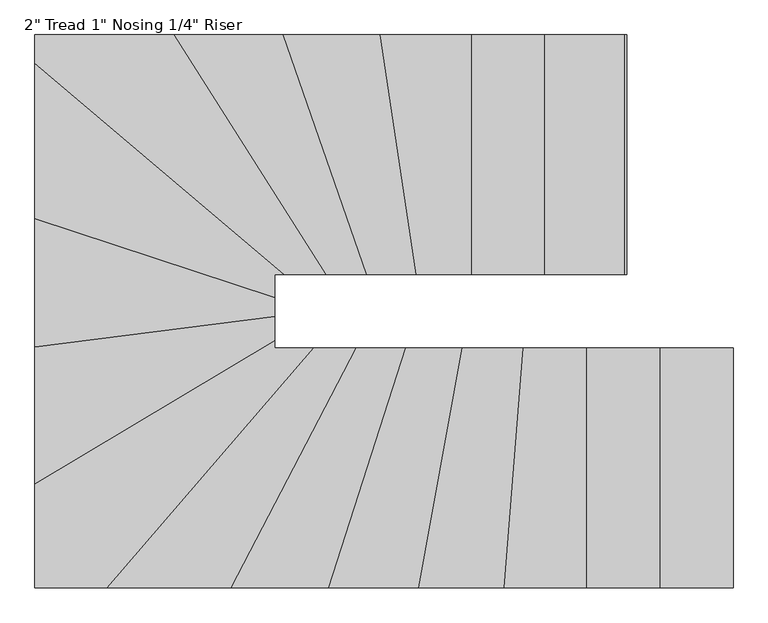
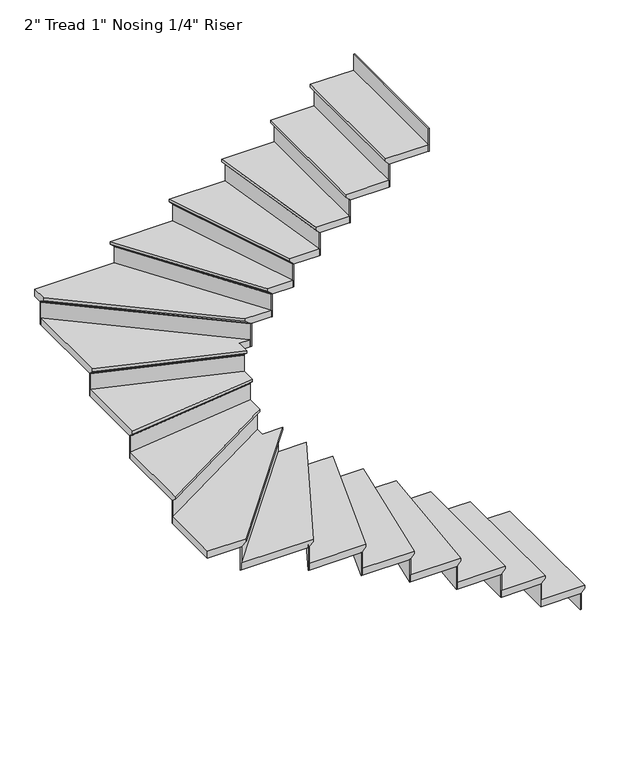
"""IFC4 building model written with IfcOpenShell, lengths in millimetres: stair flight geometry."""

from ifc_helpers import new_model, si_unit, origin, place, context, project, spatial, faceted_brep, source, transform, mapped, element, save


def stair_flight_79a896a8(model_context):
    return source(origin(), model_context, "Body", "Brep", [
        faceted_brep([(-8086.227471, 3122.5174997, 150.2833333), (-8086.227471, 3122.5174997, 169.3333333), (-8086.227471, 2208.1174997, 169.3333333), (-8086.227471, 2208.1174997, 150.2833333), (-8111.627471, 3122.5174997, 124.8833333), (-8111.627471, 2208.1174997, 124.8833333), (-8391.027471, 3122.5174997, 169.3333333), (-8391.027471, 2208.1174997, 169.3333333), (-8111.627471, 2208.1174997, 118.5333333), (-8391.027471, 2208.1174997, 118.5333333), (-8391.027471, 3122.5174997, 118.5333333), (-8111.627471, 3122.5174997, 118.5333333)], [[[0, 1, 2, 3]], [[4, 0, 3, 5]], [[2, 1, 6, 7]], [[8, 9, 10, 11]], [[2, 7, 9, 8, 5, 3]], [[8, 11, 4, 5]], [[6, 1, 0, 4, 11, 10]], [[7, 6, 10, 9]]]),
        faceted_brep([(-8111.627471, 3122.5174997, 118.5333333), (-8111.627471, 3122.5174997, 0.0), (-8117.977471, 3122.5174997, 0.0), (-8117.977471, 3122.5174997, 118.5333333), (-8111.627471, 2208.1174997, 118.5333333), (-8117.977471, 2208.1174997, 118.5333333), (-8117.977471, 2208.1174997, 0.0), (-8111.627471, 2208.1174997, 0.0)], [[[0, 1, 2, 3]], [[4, 5, 6, 7]], [[1, 0, 4, 7]], [[2, 1, 7, 6]], [[3, 2, 6, 5]], [[0, 3, 5, 4]]]),
        faceted_brep([(-8391.027471, 3122.5174997, 287.8666667), (-8391.027471, 3122.5174997, 118.5333333), (-8397.377471, 3122.5174997, 118.5333333), (-8397.377471, 3122.5174997, 287.8666667), (-8391.027471, 2208.1174997, 287.8666667), (-8397.377471, 2208.1174997, 287.8666667), (-8397.377471, 2208.1174997, 118.5333333), (-8391.027471, 2208.1174997, 118.5333333)], [[[0, 1, 2, 3]], [[4, 5, 6, 7]], [[1, 0, 4, 7]], [[2, 1, 7, 6]], [[3, 2, 6, 5]], [[0, 3, 5, 4]]]),
        faceted_brep([(-8365.627471, 2208.1174997, 338.6666667), (-8365.627471, 3122.5174997, 338.6666667), (-8670.427471, 3122.5174997, 338.6666667), (-8670.427471, 2208.1174997, 338.6666667), (-8391.027471, 2208.1174997, 287.8666667), (-8670.427471, 2208.1174997, 287.8666667), (-8670.427471, 3122.5174997, 287.8666667), (-8391.027471, 3122.5174997, 287.8666667), (-8391.027471, 2208.1174997, 294.2166667), (-8365.627471, 2208.1174997, 319.6166667), (-8391.027471, 3122.5174997, 294.2166667), (-8365.627471, 3122.5174997, 319.6166667)], [[[0, 1, 2, 3]], [[4, 5, 6, 7]], [[0, 3, 5, 4, 8, 9]], [[4, 7, 10, 8]], [[2, 1, 11, 10, 7, 6]], [[3, 2, 6, 5]], [[11, 1, 0, 9]], [[10, 11, 9, 8]]]),
        faceted_brep([(-8670.427471, 3122.5174997, 457.2), (-8670.427471, 3122.5174997, 287.8666667), (-8676.777471, 3122.5174997, 287.8666667), (-8676.777471, 3122.5174997, 457.2), (-8670.427471, 2208.1174997, 457.2), (-8676.777471, 2208.1174997, 457.2), (-8676.777471, 2208.1174997, 287.8666667), (-8670.427471, 2208.1174997, 287.8666667)], [[[0, 1, 2, 3]], [[4, 5, 6, 7]], [[1, 0, 4, 7]], [[2, 1, 7, 6]], [[3, 2, 6, 5]], [[0, 3, 5, 4]]]),
        faceted_brep([(-8645.027471, 2208.1174997, 508.0), (-8645.027471, 3122.5174997, 508.0), (-8913.9170004, 3122.5174997, 508.0), (-8985.895083, 2208.1174997, 508.0), (-8670.427471, 2208.1174997, 457.2), (-8985.895083, 2208.1174997, 457.2), (-8913.9170004, 3122.5174997, 457.2), (-8670.427471, 3122.5174997, 457.2), (-8670.427471, 2208.1174997, 463.55), (-8645.027471, 2208.1174997, 488.95), (-8670.427471, 3122.5174997, 463.55), (-8645.027471, 3122.5174997, 488.95)], [[[0, 1, 2, 3]], [[4, 5, 6, 7]], [[0, 3, 5, 4, 8, 9]], [[4, 7, 10, 8]], [[2, 1, 11, 10, 7, 6]], [[3, 2, 6, 5]], [[11, 1, 0, 9]], [[10, 11, 9, 8]]]),
        faceted_brep([(-8913.9170004, 3122.5174997, 626.5333333), (-8913.9170004, 3122.5174997, 457.2), (-8920.2866431, 3122.5174997, 457.2), (-8920.2866431, 3122.5174997, 626.5333333), (-8985.895083, 2208.1174997, 626.5333333), (-8992.2647257, 2208.1174997, 626.5333333), (-8992.2647257, 2208.1174997, 457.2), (-8985.895083, 2208.1174997, 457.2)], [[[0, 1, 2, 3]], [[4, 5, 6, 7]], [[1, 0, 4, 7]], [[2, 1, 7, 6]], [[3, 2, 6, 5]], [[0, 3, 5, 4]]]),
        faceted_brep([(-8960.4165123, 2208.1174997, 677.3333333), (-8888.4384297, 3122.5174997, 677.3333333), (-9146.6716343, 3122.5174997, 677.3333333), (-9312.6130409, 2208.1174997, 677.3333333), (-8985.895083, 2208.1174997, 626.5333333), (-9312.6130409, 2208.1174997, 626.5333333), (-9146.6716343, 3122.5174997, 626.5333333), (-8913.9170004, 3122.5174997, 626.5333333), (-8985.895083, 2208.1174997, 632.8833333), (-8960.4165123, 2208.1174997, 658.2833333), (-8913.9170004, 3122.5174997, 632.8833333), (-8888.4384297, 3122.5174997, 658.2833333)], [[[0, 1, 2, 3]], [[4, 5, 6, 7]], [[0, 3, 5, 4, 8, 9]], [[4, 7, 10, 8]], [[2, 1, 11, 10, 7, 6]], [[3, 2, 6, 5]], [[11, 1, 0, 9]], [[10, 11, 9, 8]]]),
        faceted_brep([(-9146.6716343, 3122.5174997, 795.8666667), (-9146.6716343, 3122.5174997, 626.5333333), (-9153.125351, 3122.5174997, 626.5333333), (-9153.125351, 3122.5174997, 795.8666667), (-9312.6130409, 2208.1174997, 795.8666667), (-9319.0667575, 2208.1174997, 795.8666667), (-9319.0667575, 2208.1174997, 626.5333333), (-9312.6130409, 2208.1174997, 626.5333333)], [[[0, 1, 2, 3]], [[4, 5, 6, 7]], [[1, 0, 4, 7]], [[2, 1, 7, 6]], [[3, 2, 6, 5]], [[0, 3, 5, 4]]]),
        faceted_brep([(-9286.7981743, 2208.1174997, 846.6666667), (-9120.8567677, 3122.5174997, 846.6666667), (-9363.0169479, 3122.5174997, 846.6666667), (-9656.7954295, 2208.1174997, 846.6666667), (-9312.6130409, 2208.1174997, 795.8666667), (-9656.7954295, 2208.1174997, 795.8666667), (-9363.0169479, 3122.5174997, 795.8666667), (-9146.6716343, 3122.5174997, 795.8666667), (-9312.6130409, 2208.1174997, 802.2166667), (-9286.7981743, 2208.1174997, 827.6166667), (-9146.6716343, 3122.5174997, 802.2166667), (-9120.8567677, 3122.5174997, 827.6166667)], [[[0, 1, 2, 3]], [[4, 5, 6, 7]], [[0, 3, 5, 4, 8, 9]], [[4, 7, 10, 8]], [[2, 1, 11, 10, 7, 6]], [[3, 2, 6, 5]], [[11, 1, 0, 9]], [[10, 11, 9, 8]]]),
        faceted_brep([(-9363.0169479, 3122.5174997, 965.2), (-9363.0169479, 3122.5174997, 795.8666667), (-9369.6866273, 3122.5174997, 795.8666667), (-9369.6866273, 3122.5174997, 965.2), (-9656.7954295, 2208.1174997, 965.2), (-9663.4651089, 2208.1174997, 965.2), (-9663.4651089, 2208.1174997, 795.8666667), (-9656.7954295, 2208.1174997, 795.8666667)], [[[0, 1, 2, 3]], [[4, 5, 6, 7]], [[1, 0, 4, 7]], [[2, 1, 7, 6]], [[3, 2, 6, 5]], [[0, 3, 5, 4]]]),
        faceted_brep([(-9630.1167118, 2208.1174997, 1016.0), (-9336.3382302, 3122.5174997, 1016.0), (-9552.3693579, 3122.5174997, 1016.0), (-10030.2035425, 2208.1174997, 1016.0), (-9656.7954295, 2208.1174997, 965.2), (-10030.2035425, 2208.1174997, 965.2), (-9552.3693579, 3122.5174997, 965.2), (-9363.0169479, 3122.5174997, 965.2), (-9656.7954295, 2208.1174997, 971.55), (-9630.1167118, 2208.1174997, 996.95), (-9363.0169479, 3122.5174997, 971.55), (-9336.3382302, 3122.5174997, 996.95)], [[[0, 1, 2, 3]], [[4, 5, 6, 7]], [[0, 3, 5, 4, 8, 9]], [[4, 7, 10, 8]], [[2, 1, 11, 10, 7, 6]], [[3, 2, 6, 5]], [[11, 1, 0, 9]], [[10, 11, 9, 8]]]),
        faceted_brep([(-9552.3693579, 3122.5174997, 1134.5333333), (-9552.3693579, 3122.5174997, 965.2), (-9559.5341027, 3122.5174997, 965.2), (-9559.5341027, 3122.5174997, 1134.5333333), (-10030.2035425, 2208.1174997, 1134.5333333), (-10037.3682873, 2208.1174997, 1134.5333333), (-10037.3682873, 2208.1174997, 965.2), (-10030.2035425, 2208.1174997, 965.2)], [[[0, 1, 2, 3]], [[4, 5, 6, 7]], [[1, 0, 4, 7]], [[2, 1, 7, 6]], [[3, 2, 6, 5]], [[0, 3, 5, 4]]]),
        faceted_brep([(-10001.5445633, 2208.1174997, 1185.3333333), (-9523.7103787, 3122.5174997, 1185.3333333), (-9719.9061771, 3122.5174997, 1185.3333333), (-10506.0897865, 2208.1174997, 1185.3333333), (-10030.2035425, 2208.1174997, 1134.5333333), (-10506.0897865, 2208.1174997, 1134.5333333), (-9719.9061771, 3122.5174997, 1134.5333333), (-9552.3693579, 3122.5174997, 1134.5333333), (-10030.2035425, 2208.1174997, 1140.8833333), (-10001.5445633, 2208.1174997, 1166.2833333), (-9552.3693579, 3122.5174997, 1140.8833333), (-9523.7103787, 3122.5174997, 1166.2833333)], [[[0, 1, 2, 3]], [[4, 5, 6, 7]], [[0, 3, 5, 4, 8, 9]], [[4, 7, 10, 8]], [[2, 1, 11, 10, 7, 6]], [[3, 2, 6, 5]], [[11, 1, 0, 9]], [[10, 11, 9, 8]]]),
        faceted_brep([(-9719.9061771, 3122.5174997, 1303.8666667), (-9719.9061771, 3122.5174997, 1134.5333333), (-9728.2805322, 3122.5174997, 1134.5333333), (-9728.2805322, 3122.5174997, 1303.8666667), (-10506.0897865, 2208.1174997, 1303.8666667), (-10514.4641416, 2208.1174997, 1303.8666667), (-10514.4641416, 2208.1174997, 1134.5333333), (-10506.0897865, 2208.1174997, 1134.5333333)], [[[0, 1, 2, 3]], [[4, 5, 6, 7]], [[1, 0, 4, 7]], [[2, 1, 7, 6]], [[3, 2, 6, 5]], [[0, 3, 5, 4]]]),
        faceted_brep([(-10747.2073372, 2633.5177157, 1354.6666667), (-10747.2073372, 2208.1174997, 1354.6666667), (-10472.5923659, 2208.1174997, 1354.6666667), (-9686.4087566, 3122.5174997, 1354.6666667), (-9832.8073372, 3122.5174997, 1354.6666667), (-9832.8073372, 3181.4002288, 1354.6666667), (-10747.2073372, 2208.1174997, 1303.8666667), (-10747.2073372, 2633.5177157, 1303.8666667), (-9832.8073372, 3181.4002288, 1303.8666667), (-9832.8073372, 3122.5174997, 1303.8666667), (-9719.9061771, 3122.5174997, 1303.8666667), (-10506.0897865, 2208.1174997, 1303.8666667), (-9719.9061771, 3122.5174997, 1310.2166667), (-10506.0897865, 2208.1174997, 1310.2166667), (-9686.4087566, 3122.5174997, 1335.6166667), (-10472.5923659, 2208.1174997, 1335.6166667)], [[[0, 1, 2, 3, 4, 5]], [[6, 7, 8, 9, 10, 11]], [[1, 0, 7, 6]], [[11, 10, 12, 13]], [[5, 4, 9, 8]], [[0, 5, 8, 7]], [[14, 3, 2, 15]], [[12, 14, 15, 13]], [[2, 1, 6, 11, 13, 15]], [[4, 3, 14, 12, 10, 9]]]),
        faceted_brep([(-9832.8073372, 3181.4002288, 1473.2), (-9832.8073372, 3181.4002288, 1303.8666667), (-9832.8073372, 3188.8028327, 1303.8666667), (-9832.8073372, 3188.8028327, 1473.2), (-10747.2073372, 2633.5177157, 1473.2), (-10747.2073372, 2640.9203196, 1473.2), (-10747.2073372, 2640.9203196, 1303.8666667), (-10747.2073372, 2633.5177157, 1303.8666667)], [[[0, 1, 2, 3]], [[4, 5, 6, 7]], [[1, 0, 4, 7]], [[2, 1, 7, 6]], [[3, 2, 6, 5]], [[0, 3, 5, 4]]]),
        faceted_brep([(-10747.2073372, 2603.9073003, 1524.0), (-9832.8073372, 3151.7898134, 1524.0), (-9832.8073372, 3267.6146892, 1524.0), (-10747.2073372, 3151.2124555, 1524.0), (-10747.2073372, 2633.5177157, 1473.2), (-10747.2073372, 3151.2124555, 1473.2), (-9832.8073372, 3267.6146892, 1473.2), (-9832.8073372, 3181.4002288, 1473.2), (-10747.2073372, 2633.5177157, 1479.55), (-10747.2073372, 2603.9073003, 1504.95), (-9832.8073372, 3181.4002288, 1479.55), (-9832.8073372, 3151.7898134, 1504.95)], [[[0, 1, 2, 3]], [[4, 5, 6, 7]], [[0, 3, 5, 4, 8, 9]], [[4, 7, 10, 8]], [[2, 1, 11, 10, 7, 6]], [[3, 2, 6, 5]], [[11, 1, 0, 9]], [[10, 11, 9, 8]]]),
        faceted_brep([(-9832.8073372, 3267.6146892, 1642.5333333), (-9832.8073372, 3267.6146892, 1473.2), (-9832.8073372, 3274.0159334, 1473.2), (-9832.8073372, 3274.0159334, 1642.5333333), (-10747.2073372, 3151.2124555, 1642.5333333), (-10747.2073372, 3157.6136998, 1642.5333333), (-10747.2073372, 3157.6136998, 1473.2), (-10747.2073372, 3151.2124555, 1473.2)], [[[0, 1, 2, 3]], [[4, 5, 6, 7]], [[1, 0, 4, 7]], [[2, 1, 7, 6]], [[3, 2, 6, 5]], [[0, 3, 5, 4]]]),
        faceted_brep([(-10747.2073372, 3125.6074786, 1693.3333333), (-9832.8073372, 3242.0097122, 1693.3333333), (-9832.8073372, 3340.7509196, 1693.3333333), (-10747.2073372, 3641.8025654, 1693.3333333), (-10747.2073372, 3151.2124555, 1642.5333333), (-10747.2073372, 3641.8025654, 1642.5333333), (-9832.8073372, 3340.7509196, 1642.5333333), (-9832.8073372, 3267.6146892, 1642.5333333), (-10747.2073372, 3151.2124555, 1648.8833333), (-10747.2073372, 3125.6074786, 1674.2833333), (-9832.8073372, 3267.6146892, 1648.8833333), (-9832.8073372, 3242.0097122, 1674.2833333)], [[[0, 1, 2, 3]], [[4, 5, 6, 7]], [[0, 3, 5, 4, 8, 9]], [[4, 7, 10, 8]], [[2, 1, 11, 10, 7, 6]], [[3, 2, 6, 5]], [[11, 1, 0, 9]], [[10, 11, 9, 8]]]),
        faceted_brep([(-9832.8073372, 3340.7509196, 1811.8666667), (-9832.8073372, 3340.7509196, 1642.5333333), (-9832.8073372, 3347.4362214, 1642.5333333), (-9832.8073372, 3347.4362214, 1811.8666667), (-10747.2073372, 3641.8025654, 1811.8666667), (-10747.2073372, 3648.4878672, 1811.8666667), (-10747.2073372, 3648.4878672, 1642.5333333), (-10747.2073372, 3641.8025654, 1642.5333333)], [[[0, 1, 2, 3]], [[4, 5, 6, 7]], [[1, 0, 4, 7]], [[2, 1, 7, 6]], [[3, 2, 6, 5]], [[0, 3, 5, 4]]]),
        faceted_brep([(-10747.2073372, 3615.061358, 1862.6666667), (-9832.8073372, 3314.0097122, 1862.6666667), (-9832.8073372, 3401.9174997, 1862.6666667), (-9756.9168091, 3401.9174997, 1862.6666667), (-10747.2073372, 4242.112231, 1862.6666667), (-10747.2073372, 3641.8025654, 1811.8666667), (-10747.2073372, 4242.112231, 1811.8666667), (-9756.9168091, 3401.9174997, 1811.8666667), (-9832.8073372, 3401.9174997, 1811.8666667), (-9832.8073372, 3340.7509196, 1811.8666667), (-10747.2073372, 3641.8025654, 1818.2166667), (-10747.2073372, 3615.061358, 1843.6166667), (-9832.8073372, 3340.7509196, 1818.2166667), (-9832.8073372, 3314.0097122, 1843.6166667)], [[[0, 1, 2, 3, 4]], [[5, 6, 7, 8, 9]], [[0, 4, 6, 5, 10, 11]], [[5, 9, 12, 10]], [[2, 1, 13, 12, 9, 8]], [[4, 3, 7, 6]], [[13, 1, 0, 11]], [[12, 13, 11, 10]], [[3, 2, 8, 7]]]),
        faceted_brep([(-9756.9168091, 3401.9174997, 1981.2), (-9756.9168091, 3401.9174997, 1811.8666667), (-9747.1015867, 3401.9174997, 1811.8666667), (-9747.1015867, 3401.9174997, 1981.2), (-10747.2073372, 4242.112231, 1981.2), (-10747.2073372, 4250.4397852, 1981.2), (-10747.2073372, 4250.4397852, 1811.8666667), (-10747.2073372, 4242.112231, 1811.8666667)], [[[0, 1, 2, 3]], [[4, 5, 6, 7]], [[1, 0, 4, 7]], [[2, 1, 7, 6]], [[3, 2, 6, 5]], [[0, 3, 5, 4]]]),
        faceted_brep([(-10185.8825098, 4316.3174997, 2032.0), (-10747.2073372, 4316.3174997, 2032.0), (-10747.2073372, 4208.8020138, 2032.0), (-9796.1776986, 3401.9174997, 2032.0), (-9607.0675829, 3401.9174997, 2032.0), (-10747.2073372, 4316.3174997, 1981.2), (-10185.8825098, 4316.3174997, 1981.2), (-9607.0675829, 3401.9174997, 1981.2), (-9756.9168091, 3401.9174997, 1981.2), (-10747.2073372, 4242.112231, 1981.2), (-9756.9168091, 3401.9174997, 1987.55), (-10747.2073372, 4242.112231, 1987.55), (-9796.1776986, 3401.9174997, 2012.95), (-10747.2073372, 4208.8020138, 2012.95)], [[[0, 1, 2, 3, 4]], [[5, 6, 7, 8, 9]], [[1, 0, 6, 5]], [[9, 8, 10, 11]], [[4, 3, 12, 10, 8, 7]], [[0, 4, 7, 6]], [[12, 3, 2, 13]], [[10, 12, 13, 11]], [[2, 1, 5, 9, 11, 13]]]),
        faceted_brep([(-9607.0675829, 3401.9174997, 2150.5333333), (-9607.0675829, 3401.9174997, 1981.2), (-9599.552314, 3401.9174997, 1981.2), (-9599.552314, 3401.9174997, 2150.5333333), (-10185.8825098, 4316.3174997, 2150.5333333), (-10178.3672409, 4316.3174997, 2150.5333333), (-10178.3672409, 4316.3174997, 1981.2), (-10185.8825098, 4316.3174997, 1981.2)], [[[0, 1, 2, 3]], [[4, 5, 6, 7]], [[1, 0, 4, 7]], [[2, 1, 7, 6]], [[3, 2, 6, 5]], [[0, 3, 5, 4]]]),
        faceted_brep([(-10215.9435855, 4316.3174997, 2201.3333333), (-9637.1286586, 3401.9174997, 2201.3333333), (-9455.5314169, 3401.9174997, 2201.3333333), (-9774.3141998, 4316.3174997, 2201.3333333), (-10185.8825098, 4316.3174997, 2150.5333333), (-9774.3141998, 4316.3174997, 2150.5333333), (-9455.5314169, 3401.9174997, 2150.5333333), (-9607.0675829, 3401.9174997, 2150.5333333), (-10185.8825098, 4316.3174997, 2156.8833333), (-10215.9435855, 4316.3174997, 2182.2833333), (-9607.0675829, 3401.9174997, 2156.8833333), (-9637.1286586, 3401.9174997, 2182.2833333)], [[[0, 1, 2, 3]], [[4, 5, 6, 7]], [[0, 3, 5, 4, 8, 9]], [[4, 7, 10, 8]], [[2, 1, 11, 10, 7, 6]], [[3, 2, 6, 5]], [[11, 1, 0, 9]], [[10, 11, 9, 8]]]),
        faceted_brep([(-9455.5314169, 3401.9174997, 2319.8666667), (-9455.5314169, 3401.9174997, 2150.5333333), (-9448.8065916, 3401.9174997, 2150.5333333), (-9448.8065916, 3401.9174997, 2319.8666667), (-9774.3141998, 4316.3174997, 2319.8666667), (-9767.5893746, 4316.3174997, 2319.8666667), (-9767.5893746, 4316.3174997, 2150.5333333), (-9774.3141998, 4316.3174997, 2150.5333333)], [[[0, 1, 2, 3]], [[4, 5, 6, 7]], [[1, 0, 4, 7]], [[2, 1, 7, 6]], [[3, 2, 6, 5]], [[0, 3, 5, 4]]]),
        faceted_brep([(-9801.2135008, 4316.3174997, 2370.6666667), (-9482.4307179, 3401.9174997, 2370.6666667), (-9268.5456464, 3401.9174997, 2370.6666667), (-9404.936572, 4316.3174997, 2370.6666667), (-9774.3141998, 4316.3174997, 2319.8666667), (-9404.936572, 4316.3174997, 2319.8666667), (-9268.5456464, 3401.9174997, 2319.8666667), (-9455.5314169, 3401.9174997, 2319.8666667), (-9774.3141998, 4316.3174997, 2326.2166667), (-9801.2135008, 4316.3174997, 2351.6166667), (-9455.5314169, 3401.9174997, 2326.2166667), (-9482.4307179, 3401.9174997, 2351.6166667)], [[[0, 1, 2, 3]], [[4, 5, 6, 7]], [[0, 3, 5, 4, 8, 9]], [[4, 7, 10, 8]], [[2, 1, 11, 10, 7, 6]], [[3, 2, 6, 5]], [[11, 1, 0, 9]], [[10, 11, 9, 8]]]),
        faceted_brep([(-9268.5456464, 3401.9174997, 2489.2), (-9268.5456464, 3401.9174997, 2319.8666667), (-9262.1253964, 3401.9174997, 2319.8666667), (-9262.1253964, 3401.9174997, 2489.2), (-9404.936572, 4316.3174997, 2489.2), (-9398.5163219, 4316.3174997, 2489.2), (-9398.5163219, 4316.3174997, 2319.8666667), (-9404.936572, 4316.3174997, 2319.8666667)], [[[0, 1, 2, 3]], [[4, 5, 6, 7]], [[1, 0, 4, 7]], [[2, 1, 7, 6]], [[3, 2, 6, 5]], [[0, 3, 5, 4]]]),
        faceted_brep([(-9430.6175721, 4316.3174997, 2540.0), (-9294.2266465, 3401.9174997, 2540.0), (-9057.6221093, 3401.9174997, 2540.0), (-9057.6221093, 4316.3174997, 2540.0), (-9404.936572, 4316.3174997, 2489.2), (-9057.6221093, 4316.3174997, 2489.2), (-9057.6221093, 3401.9174997, 2489.2), (-9268.5456464, 3401.9174997, 2489.2), (-9404.936572, 4316.3174997, 2495.55), (-9430.6175721, 4316.3174997, 2520.95), (-9268.5456464, 3401.9174997, 2495.55), (-9294.2266465, 3401.9174997, 2520.95)], [[[0, 1, 2, 3]], [[4, 5, 6, 7]], [[0, 3, 5, 4, 8, 9]], [[4, 7, 10, 8]], [[2, 1, 11, 10, 7, 6]], [[3, 2, 6, 5]], [[11, 1, 0, 9]], [[10, 11, 9, 8]]]),
        faceted_brep([(-9057.6221093, 3401.9174997, 2658.5333333), (-9057.6221093, 3401.9174997, 2489.2), (-9051.2721093, 3401.9174997, 2489.2), (-9051.2721093, 3401.9174997, 2658.5333333), (-9057.6221093, 4316.3174997, 2658.5333333), (-9051.2721093, 4316.3174997, 2658.5333333), (-9051.2721093, 4316.3174997, 2489.2), (-9057.6221093, 4316.3174997, 2489.2)], [[[0, 1, 2, 3]], [[4, 5, 6, 7]], [[1, 0, 4, 7]], [[2, 1, 7, 6]], [[3, 2, 6, 5]], [[0, 3, 5, 4]]]),
        faceted_brep([(-9083.0221093, 4316.3174997, 2709.3333333), (-9083.0221093, 3401.9174997, 2709.3333333), (-8778.2221093, 3401.9174997, 2709.3333333), (-8778.2221093, 4316.3174997, 2709.3333333), (-9057.6221093, 4316.3174997, 2658.5333333), (-8778.2221093, 4316.3174997, 2658.5333333), (-8778.2221093, 3401.9174997, 2658.5333333), (-9057.6221093, 3401.9174997, 2658.5333333), (-9057.6221093, 4316.3174997, 2664.8833333), (-9083.0221093, 4316.3174997, 2690.2833333), (-9057.6221093, 3401.9174997, 2664.8833333), (-9083.0221093, 3401.9174997, 2690.2833333)], [[[0, 1, 2, 3]], [[4, 5, 6, 7]], [[0, 3, 5, 4, 8, 9]], [[4, 7, 10, 8]], [[2, 1, 11, 10, 7, 6]], [[3, 2, 6, 5]], [[11, 1, 0, 9]], [[10, 11, 9, 8]]]),
        faceted_brep([(-8778.2221093, 3401.9174997, 2827.8666667), (-8778.2221093, 3401.9174997, 2658.5333333), (-8771.8721093, 3401.9174997, 2658.5333333), (-8771.8721093, 3401.9174997, 2827.8666667), (-8778.2221093, 4316.3174997, 2827.8666667), (-8771.8721093, 4316.3174997, 2827.8666667), (-8771.8721093, 4316.3174997, 2658.5333333), (-8778.2221093, 4316.3174997, 2658.5333333)], [[[0, 1, 2, 3]], [[4, 5, 6, 7]], [[1, 0, 4, 7]], [[2, 1, 7, 6]], [[3, 2, 6, 5]], [[0, 3, 5, 4]]]),
        faceted_brep([(-8498.8221093, 3401.9174997, 2997.2), (-8498.8221093, 3401.9174997, 2827.8666667), (-8492.4721093, 3401.9174997, 2827.8666667), (-8492.4721093, 3401.9174997, 2997.2), (-8498.8221093, 4316.3174997, 2997.2), (-8492.4721093, 4316.3174997, 2997.2), (-8492.4721093, 4316.3174997, 2827.8666667), (-8498.8221093, 4316.3174997, 2827.8666667)], [[[0, 1, 2, 3]], [[4, 5, 6, 7]], [[1, 0, 4, 7]], [[2, 1, 7, 6]], [[3, 2, 6, 5]], [[0, 3, 5, 4]]]),
        faceted_brep([(-8803.6221093, 4316.3174997, 2878.6666667), (-8803.6221093, 3401.9174997, 2878.6666667), (-8498.8221093, 3401.9174997, 2878.6666667), (-8498.8221093, 4316.3174997, 2878.6666667), (-8778.2221093, 4316.3174997, 2827.8666667), (-8498.8221093, 4316.3174997, 2827.8666667), (-8498.8221093, 3401.9174997, 2827.8666667), (-8778.2221093, 3401.9174997, 2827.8666667), (-8778.2221093, 4316.3174997, 2834.2166667), (-8803.6221093, 4316.3174997, 2859.6166667), (-8778.2221093, 3401.9174997, 2834.2166667), (-8803.6221093, 3401.9174997, 2859.6166667)], [[[0, 1, 2, 3]], [[4, 5, 6, 7]], [[0, 3, 5, 4, 8, 9]], [[4, 7, 10, 8]], [[2, 1, 11, 10, 7, 6]], [[3, 2, 6, 5]], [[11, 1, 0, 9]], [[10, 11, 9, 8]]]),
    ])


if __name__ == "__main__":
    model = new_model("IFC4")
    model_context = context("Model", 3, world=origin())
    ifc_project = project(units=[si_unit("LENGTHUNIT", "METRE", prefix="MILLI")], contexts=[model_context])
    site = spatial("IfcSite", under=ifc_project)
    building = spatial("IfcBuilding", under=site)
    placement = place(None, origin())
    stair_flight_shape = stair_flight_79a896a8(model_context)
    element("IfcStairFlight", 1, ObjectType="2\" Tread 1\" Nosing 1/4\" Riser", at=placement, inside=building, context=model_context, shape_type="MappedRepresentation", body=[
        mapped(stair_flight_shape, transform((0.0, 0.0, 0.0), x_axis=(1.0, 0.0, 0.0), y_axis=(0.0, 1.0, 0.0), z_axis=(0.0, 0.0, 1.0))),
    ])
    save(model, "model.ifc")
